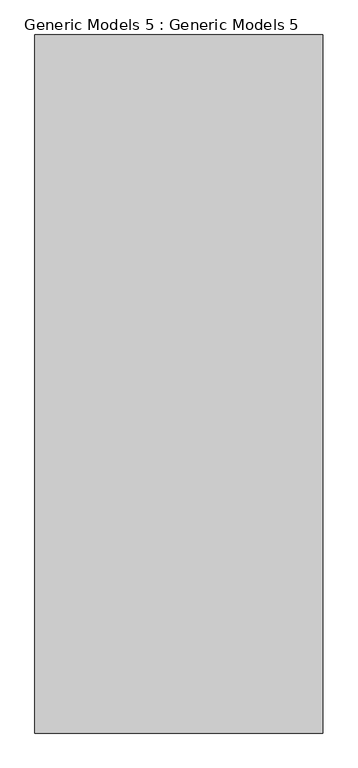
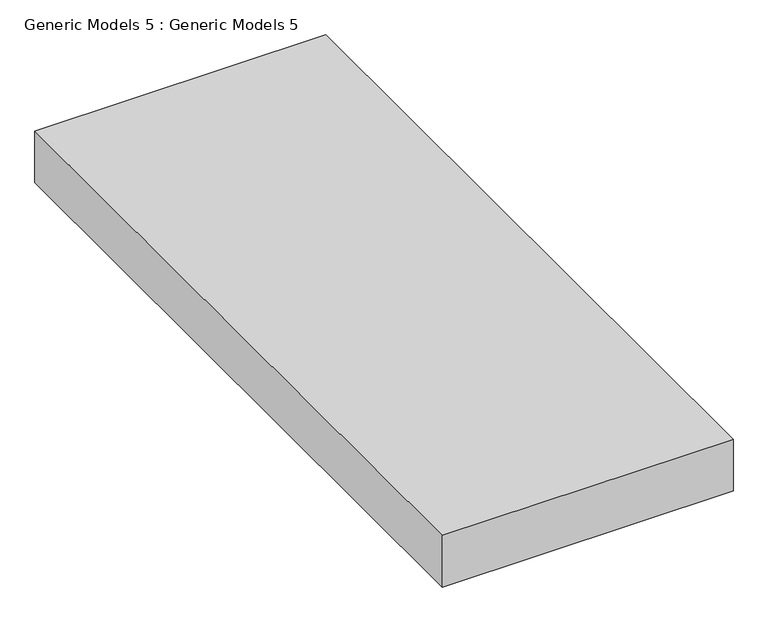
"""IFC4 building model written with IfcOpenShell, lengths in millimetres: proxy geometry, Generic Models 5 : Generic Models 5."""

from ifc_helpers import new_model, si_unit, frame, origin, place, context, project, spatial, polyline, outline, extrude, source, transform, mapped, element, save


def generic_models_5_generic_models_5_11858d31(model_context):
    return source(origin(), model_context, "Body", "SweptSolid", [
        extrude(outline(polyline([(-4652.2120831, -403.4023776), (-5871.4120831, -403.4023776), (-5871.4120831, 2555.2054373), (-4652.2120831, 2555.2054373), (-4652.2120831, -403.4023776)])), frame((0.0, 0.0, 2338.9510739), z_axis=(0.0, 0.0, 1.0), x_axis=(1.0, 0.0, 0.0)), (0.0, 0.0, 1.0), 228.6),
    ])


if __name__ == "__main__":
    model = new_model("IFC4")
    model_context = context("Model", 3, world=origin())
    ifc_project = project(units=[si_unit("LENGTHUNIT", "METRE", prefix="MILLI")], contexts=[model_context])
    site = spatial("IfcSite", under=ifc_project)
    building = spatial("IfcBuilding", under=site)
    placement = place(None, origin())
    generic_models_5_generic_models_5_shape = generic_models_5_generic_models_5_11858d31(model_context)
    element("IfcBuildingElementProxy", 1, Name="Generic Models 5 : Generic Models 5", ObjectType="Generic Models 5 : Generic Models 5", at=placement, inside=building, context=model_context, shape_type="MappedRepresentation", body=[
        mapped(generic_models_5_generic_models_5_shape, transform((0.0, 0.0, 0.0), x_axis=(1.0, 0.0, 0.0), y_axis=(0.0, 1.0, 0.0), z_axis=(0.0, 0.0, 1.0))),
    ])
    save(model, "model.ifc")
